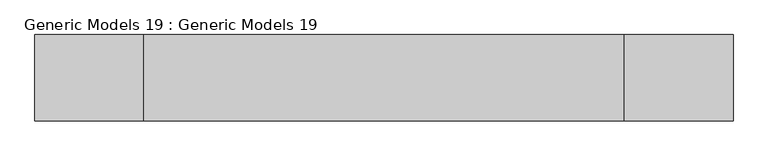
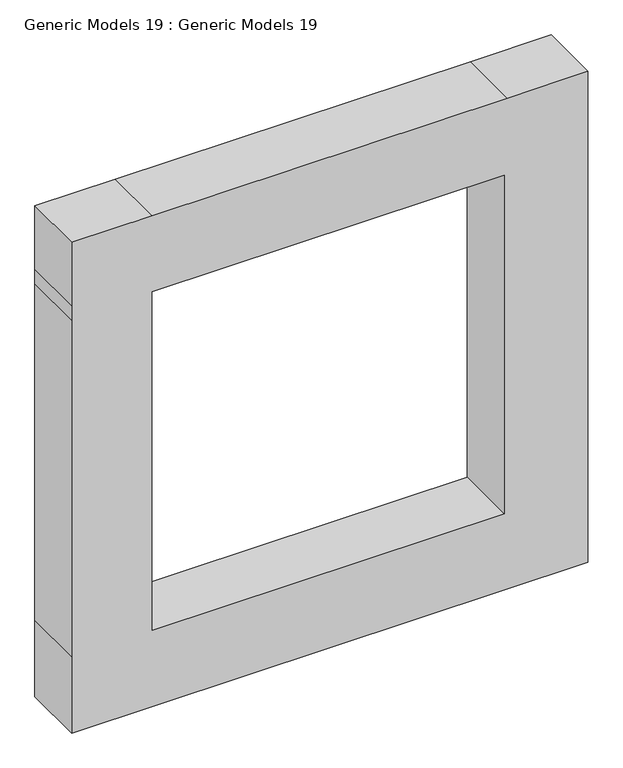
"""IFC4 building model written with IfcOpenShell, lengths in millimetres: proxy geometry, Generic Models 19 : Generic Models 19."""

from ifc_helpers import new_model, si_unit, frame, origin, place, context, project, spatial, polyline, outline, extrude, source, transform, mapped, element, save


def generic_models_19_generic_models_19_60db133f(model_context):
    return source(origin(), model_context, "Body", "SweptSolid", [
        extrude(outline(polyline([(2181.2676291, 4320.9463194), (835.0676291, 4320.9463194), (530.2676291, 4320.9463194), (530.2676291, 6276.7463194), (835.0676291, 6276.7463194), (2495.55, 6276.7463194), (2495.55, 5971.9463194), (2495.55, 4625.7463194), (2495.55, 4320.9463194), (2241.55, 4320.9463194), (2181.2676291, 4320.9463194)]), holes=[polyline([(2190.75, 5959.2463194), (835.0676291, 5959.2463194), (835.0676291, 4625.7463194), (2190.75, 4625.7463194), (2190.75, 5959.2463194)])]), frame((0.0, -4112.712639, 0.0), z_axis=(0.0, 1.0, 0.0), x_axis=(0.0, 0.0, 1.0)), (0.0, 0.0, 1.0), 241.1853288),
    ])


if __name__ == "__main__":
    model = new_model("IFC4")
    model_context = context("Model", 3, world=origin())
    ifc_project = project(units=[si_unit("LENGTHUNIT", "METRE", prefix="MILLI")], contexts=[model_context])
    site = spatial("IfcSite", under=ifc_project)
    building = spatial("IfcBuilding", under=site)
    placement = place(None, origin())
    generic_models_19_generic_models_19_shape = generic_models_19_generic_models_19_60db133f(model_context)
    element("IfcBuildingElementProxy", 1, Name="Generic Models 19 : Generic Models 19", ObjectType="Generic Models 19 : Generic Models 19", at=placement, inside=building, context=model_context, shape_type="MappedRepresentation", body=[
        mapped(generic_models_19_generic_models_19_shape, transform((0.0, 0.0, 0.0), x_axis=(1.0, 0.0, 0.0), y_axis=(0.0, 1.0, 0.0), z_axis=(0.0, 0.0, 1.0))),
    ])
    save(model, "model.ifc")

# Revit data of these elements
# Element 1 (IfcBuildingElementProxy, "Generic Models 19 : Generic Models 19")
#   Materials on its faces: "exterior wall"
# Materials
#   "exterior wall": class "Generic", colour RGB 215 217 121, transparency 0, Cost = 0
